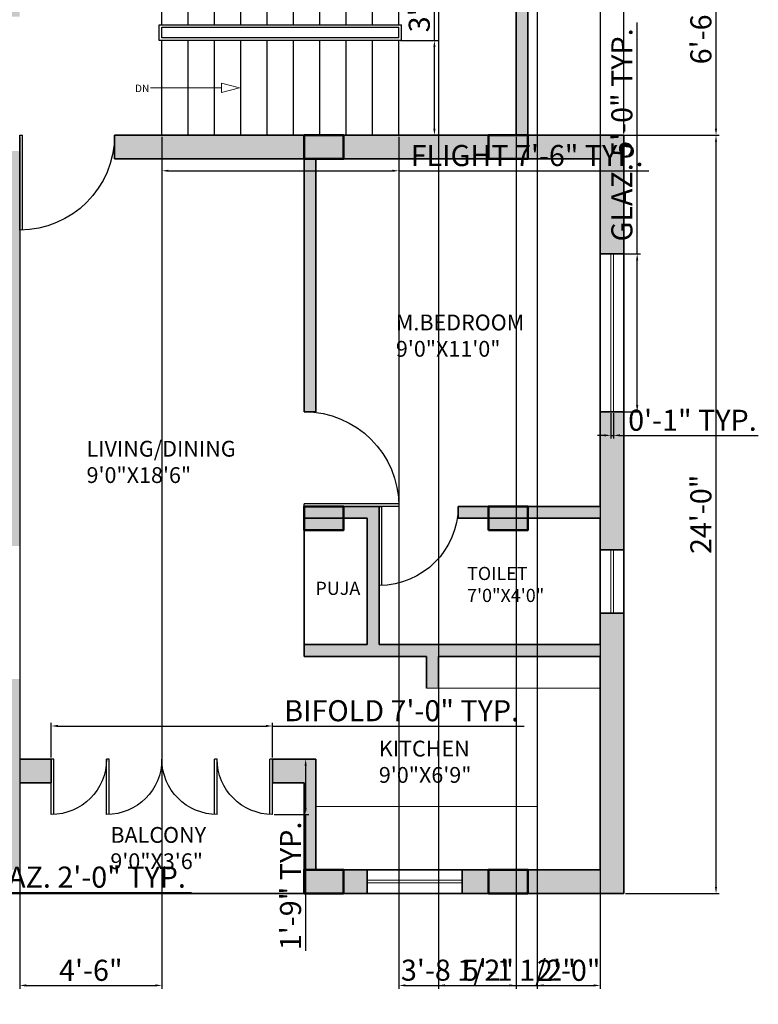
# Model space of a CAD drawing. Units: inches. Extents: x 3010 to 3575, y 2253 to 2995.
# Tile 2 of 4: x 3258 to 3538, y 2253 to 2627. Entities that reach past the tile are written whole.
import ezdxf

# ---------------------------------------------------------------- set-up
doc = ezdxf.new("R2010")
doc.units = ezdxf.units.IN
for name, color, linetype, lineweight in [('A-ANNO-DIMS', 2, 'Continuous', 18), ('A-ANNO-SYMB', 7, 'Continuous', 18), ('A-ANNO-TEXT', 7, 'Continuous', 18), ('A-AREA-IDEN', 7, 'Continuous', 18), ('A-COLS', 7, 'Continuous', 50), ('A-COLS-PATT', 1, 'Continuous', 13), ('A-DOOR', 3, 'Continuous', 25), ('A-FLOR-FIXT', 8, 'Continuous', 18), ('A-FLOR-STRS', 7, 'Continuous', 25), ('A-GLAZ', 4, 'Continuous', 18), ('A-WALL', 7, 'Continuous', 35)]:
    doc.layers.add(name, color=color, linetype=linetype, lineweight=lineweight)
doc.layers.add('A-WALL-PATT', color=9, linetype='Continuous', lineweight=13, true_color=0xc7c8ca)
doc.styles.get("Standard").update_dxf_attribs({"font": 'arial.ttf'})
doc.dimstyles.new('ISO-25', dxfattribs={"dimtxt": 8, "dimasz": 2.5, "dimexe": 1.25, "dimexo": 0.625, "dimtad": 1, "dimdec": 1, "dimlunit": 3, "dimtxsty": 'Standard', "dimcen": 2.5, "dimadec": 0, "dimazin": 0, "dimtfac": 1, "dimtdec": 1, "dimtmove": 0, "dimatfit": 3, "dimfxl": 1, "dimarcsym": 0})

# ---------------------------------------------------------------- blocks, each defined once
blk = doc.blocks.new("D1 3'")
for p, q in [((0, 36), (0, 0)), ((1, 36), (1, 0)), ((0, 0), (1, 0))]:
    blk.add_line(p, q)
blk.add_arc((0, 0), 36, 0, 90)
blk = doc.blocks.new("D2 2'6")
for p, q in [((0, 30), (0, 0)), ((1, 30), (1, 0)), ((0, 0), (1, 0))]:
    blk.add_line(p, q)
blk.add_arc((0, 0), 30, 0, 90)
blk = doc.blocks.new('FLOD D')
for p, q in [((3539.49, 2401.61), (3539.49, 2380.61)), ((3540.49, 2401.61), (3540.49, 2380.61)), ((3560.49, 2401.61), (3560.49, 2380.61)), ((3561.49, 2401.61), (3561.49, 2380.61)), ((3601.49, 2401.61), (3601.49, 2380.61)), ((3602.49, 2401.61), (3602.49, 2380.61)), ((3622.49, 2401.61), (3622.49, 2380.61)), ((3623.49, 2401.61), (3623.49, 2380.61)), ((3540.49, 2380.61), (3539.49, 2380.61)), ((3561.49, 2380.61), (3560.49, 2380.61)), ((3602.49, 2380.61), (3601.49, 2380.61)), ((3623.49, 2380.61), (3622.49, 2380.61))]:
    blk.add_line(p, q)
for centre, start, end in [((3539.49, 2380.61), 0, 90), ((3560.49, 2380.61), 0, 90), ((3602.49, 2380.61), 90, 180), ((3623.49, 2380.61), 90, 180)]:
    blk.add_arc(centre, 21, start, end)
blk = doc.blocks.new('GLAZING-24IN')
for p, q in [((24, 1), (0, 1)), ((24, 0), (0, 0))]:
    blk.add_line(p, q)
blk = doc.blocks.new('GLAZING-36IN')
for p, q in [((36, 1), (0, 1)), ((36, 0), (0, 0))]:
    blk.add_line(p, q)
blk = doc.blocks.new('GLAZING-60IN')
for p, q in [((0, 0), (0, 60)), ((1, 0), (1, 60))]:
    blk.add_line(p, q)
blk = doc.blocks.new('STAIR-FLIGHT-36IN')
for p, q in [((0, 0), (0, 36)), ((10, 0), (10, 36)), ((20, 0), (20, 36)), ((30, 0), (30, 36)), ((40, 0), (40, 36)), ((50, 0), (50, 36)), ((60, 0), (60, 36)), ((70, 0), (70, 36)), ((80, 0), (80, 36)), ((90, 0), (90, 36))]:
    blk.add_line(p, q)
blk = doc.blocks.new('STAIR-DIRECTION-ARROW')
blk.add_line((0, 1.77), (26.94, 1.77))
blk.add_lwpolyline([(33.73, 1.77), (26.94, 3.54), (26.94, 0)], close=True)
blk = doc.blocks.new('KITCHEN-COUNTER-L')
for p, q in [((84, 45), (84, 0)), ((84, 0), (0, 0))]:
    blk.add_line(p, q)
blk = doc.blocks.new('*D17')
at = {"layer": 'A-ANNO-DIMS', "color": 0, "lineweight": -2, "transparency": 16777216}
for p, q in [((3211.45, 2298.76), (3211.45, 2294.53)), ((3235.45, 2298.76), (3235.45, 2294.53)), ((3213.95, 2295.78), (3232.95, 2295.78)), ((3235.45, 2295.78), (3323.23, 2295.78))]:
    blk.add_line(p, q, dxfattribs=at)
at = {"layer": 'A-ANNO-DIMS', "color": 0, "transparency": 16777216}
for points in [[(3213.95, 2296.2), (3213.95, 2295.37), (3211.45, 2295.78)], [(3232.95, 2296.2), (3232.95, 2295.37), (3235.45, 2295.78)]]:
    blk.add_solid(points, dxfattribs=at)
at = {"layer": 'Defpoints', "color": 0, "transparency": 16777216}
for p in [(3211.45, 2299.38), (3235.45, 2299.38), (3235.45, 2295.78)]:
    blk.add_point(p, dxfattribs=at)
at = {"layer": 'A-ANNO-DIMS', "color": 0, "transparency": 16777216, "insert": (3280.59, 2300.54), "char_height": 8, "attachment_point": 5}
blk.add_mtext('GLAZ. 2\'-0" TYP.', dxfattribs=at)
blk = doc.blocks.new('*D21')
at = {"layer": 'A-ANNO-DIMS', "color": 0, "lineweight": -2, "transparency": 16777216}
for p, q in [((3492.45, 2538.38), (3492.45, 2626.17)), ((3484.07, 2538.38), (3493.7, 2538.38)), ((3492.45, 2480.88), (3492.45, 2535.88)), ((3484.07, 2478.38), (3493.7, 2478.38))]:
    blk.add_line(p, q, dxfattribs=at)
at = {"layer": 'A-ANNO-DIMS', "color": 0, "transparency": 16777216}
for points in [[(3492.03, 2535.88), (3492.86, 2535.88), (3492.45, 2538.38)], [(3492.03, 2480.88), (3492.86, 2480.88), (3492.45, 2478.38)]]:
    blk.add_solid(points, dxfattribs=at)
at = {"layer": 'Defpoints', "color": 0, "transparency": 16777216}
for p in [(3483.45, 2538.38), (3492.45, 2538.38), (3483.45, 2478.38)]:
    blk.add_point(p, dxfattribs=at)
at = {"layer": 'A-ANNO-DIMS', "color": 0, "transparency": 16777216, "insert": (3487.68, 2583.52), "char_height": 8, "attachment_point": 5, "rotation": 90}
blk.add_mtext('GLAZ. 5\'-0" TYP.', dxfattribs=at)
blk = doc.blocks.new('*D22')
at = {"layer": 'A-ANNO-DIMS', "color": 0, "lineweight": -2, "transparency": 16777216}
for p, q in [((3482.45, 2477.76), (3482.45, 2468.13)), ((3483.45, 2477.76), (3483.45, 2468.13)), ((3479.95, 2469.38), (3477.45, 2469.38)), ((3482.45, 2469.38), (3483.45, 2469.38)), ((3485.95, 2469.38), (3538.46, 2469.38))]:
    blk.add_line(p, q, dxfattribs=at)
at = {"layer": 'A-ANNO-DIMS', "color": 0, "transparency": 16777216}
for points in [[(3479.95, 2469.8), (3479.95, 2468.97), (3482.45, 2469.38)], [(3485.95, 2469.8), (3485.95, 2468.97), (3483.45, 2469.38)]]:
    blk.add_solid(points, dxfattribs=at)
at = {"layer": 'Defpoints', "color": 0, "transparency": 16777216}
for p in [(3482.45, 2478.38), (3483.45, 2478.38), (3483.45, 2469.38)]:
    blk.add_point(p, dxfattribs=at)
at = {"layer": 'A-ANNO-DIMS', "color": 0, "transparency": 16777216, "insert": (3513.45, 2474.09), "char_height": 8, "attachment_point": 5}
blk.add_mtext('0\'-1" TYP.', dxfattribs=at)
blk = doc.blocks.new('*D29')
at = {"layer": 'A-ANNO-DIMS', "color": 0, "lineweight": -2, "transparency": 16777216}
for p, q in [((3269.95, 2347.01), (3269.95, 2360.23)), ((3353.95, 2347.01), (3353.95, 2360.23)), ((3272.45, 2358.98), (3351.45, 2358.98)), ((3353.95, 2358.98), (3449.58, 2358.98))]:
    blk.add_line(p, q, dxfattribs=at)
at = {"layer": 'A-ANNO-DIMS', "color": 0, "transparency": 16777216}
for points in [[(3272.45, 2359.4), (3272.45, 2358.57), (3269.95, 2358.98)], [(3351.45, 2359.4), (3351.45, 2358.57), (3353.95, 2358.98)]]:
    blk.add_solid(points, dxfattribs=at)
at = {"layer": 'Defpoints', "color": 0, "transparency": 16777216}
for p in [(3353.95, 2358.98), (3269.95, 2346.38), (3353.95, 2346.38)]:
    blk.add_point(p, dxfattribs=at)
at = {"layer": 'A-ANNO-DIMS', "color": 0, "transparency": 16777216, "insert": (3403.01, 2363.75), "char_height": 8, "attachment_point": 5}
blk.add_mtext('BIFOLD 7\'-0" TYP.', dxfattribs=at)
blk = doc.blocks.new('*D30')
at = {"layer": 'A-ANNO-DIMS', "color": 0, "lineweight": -2, "transparency": 16777216}
for p, q in [((3354.57, 2346.38), (3367.8, 2346.38)), ((3366.55, 2343.88), (3366.55, 2327.88)), ((3354.57, 2325.38), (3367.8, 2325.38)), ((3366.55, 2325.38), (3366.55, 2273.62))]:
    blk.add_line(p, q, dxfattribs=at)
at = {"layer": 'A-ANNO-DIMS', "color": 0, "transparency": 16777216}
for points in [[(3366.13, 2343.88), (3366.96, 2343.88), (3366.55, 2346.38)], [(3366.13, 2327.88), (3366.96, 2327.88), (3366.55, 2325.38)]]:
    blk.add_solid(points, dxfattribs=at)
at = {"layer": 'Defpoints', "color": 0, "transparency": 16777216}
for p in [(3353.95, 2346.38), (3353.95, 2325.38), (3366.55, 2325.38)]:
    blk.add_point(p, dxfattribs=at)
at = {"layer": 'A-ANNO-DIMS', "color": 0, "transparency": 16777216, "insert": (3361.84, 2298.25), "char_height": 8, "attachment_point": 5, "rotation": 90}
blk.add_mtext('1\'-9" TYP.', dxfattribs=at)
blk = doc.blocks.new('*D33')
at = {"layer": 'A-ANNO-DIMS', "color": 0, "lineweight": -2, "transparency": 16777216}
for p, q in [((3311.95, 2582.76), (3311.95, 2568.63)), ((3401.95, 2582.76), (3401.95, 2568.63)), ((3314.45, 2569.88), (3399.45, 2569.88)), ((3401.95, 2569.88), (3496.85, 2569.88))]:
    blk.add_line(p, q, dxfattribs=at)
at = {"layer": 'A-ANNO-DIMS', "color": 0, "transparency": 16777216}
for points in [[(3314.45, 2570.3), (3314.45, 2569.47), (3311.95, 2569.88)], [(3399.45, 2570.3), (3399.45, 2569.47), (3401.95, 2569.88)]]:
    blk.add_solid(points, dxfattribs=at)
at = {"layer": 'Defpoints', "color": 0, "transparency": 16777216}
for p in [(3311.95, 2583.38), (3401.95, 2583.38), (3401.95, 2569.88)]:
    blk.add_point(p, dxfattribs=at)
at = {"layer": 'A-ANNO-DIMS', "color": 0, "transparency": 16777216, "insert": (3450.65, 2574.64), "char_height": 8, "attachment_point": 5}
blk.add_mtext('FLIGHT 7\'-6" TYP.', dxfattribs=at)
blk = doc.blocks.new('*D34')
at = {"layer": 'A-ANNO-DIMS', "color": 0, "lineweight": -2, "transparency": 16777216}
for p, q in [((3415.45, 2619.38), (3415.45, 2671.89)), ((3402.57, 2619.38), (3416.7, 2619.38)), ((3415.45, 2585.88), (3415.45, 2616.88)), ((3402.57, 2583.38), (3416.7, 2583.38))]:
    blk.add_line(p, q, dxfattribs=at)
at = {"layer": 'A-ANNO-DIMS', "color": 0, "transparency": 16777216}
for points in [[(3415.03, 2616.88), (3415.86, 2616.88), (3415.45, 2619.38)], [(3415.03, 2585.88), (3415.86, 2585.88), (3415.45, 2583.38)]]:
    blk.add_solid(points, dxfattribs=at)
at = {"layer": 'Defpoints', "color": 0, "transparency": 16777216}
for p in [(3401.95, 2619.38), (3415.45, 2619.38), (3401.95, 2583.38)]:
    blk.add_point(p, dxfattribs=at)
at = {"layer": 'A-ANNO-DIMS', "color": 0, "transparency": 16777216, "insert": (3410.73, 2646.89), "char_height": 8, "attachment_point": 5, "rotation": 90}
blk.add_mtext('3\'-0" TYP.', dxfattribs=at)
blk = doc.blocks.new('*D35')
at = {"layer": 'A-ANNO-DIMS', "color": 0, "lineweight": -2, "transparency": 16777216}
for p, q in [((3257.95, 2582.76), (3257.95, 2259.18)), ((3311.95, 2582.76), (3311.95, 2259.18)), ((3260.45, 2260.43), (3309.45, 2260.43))]:
    blk.add_line(p, q, dxfattribs=at)
at = {"layer": 'A-ANNO-DIMS', "color": 0, "transparency": 16777216}
for points in [[(3260.45, 2260.85), (3260.45, 2260.02), (3257.95, 2260.43)], [(3309.45, 2260.85), (3309.45, 2260.02), (3311.95, 2260.43)]]:
    blk.add_solid(points, dxfattribs=at)
at = {"layer": 'Defpoints', "color": 0, "transparency": 16777216}
for p in [(3257.95, 2583.38), (3311.95, 2583.38), (3311.95, 2260.43)]:
    blk.add_point(p, dxfattribs=at)
at = {"layer": 'A-ANNO-DIMS', "color": 0, "transparency": 16777216, "insert": (3284.95, 2265.14), "char_height": 8, "attachment_point": 5}
blk.add_mtext('4\'-6"', dxfattribs=at)
blk = doc.blocks.new('*D36')
at = {"layer": 'A-ANNO-DIMS', "color": 0, "lineweight": -2, "transparency": 16777216}
for p, q in [((3401.95, 2582.76), (3401.95, 2259.18)), ((3446.45, 2582.76), (3446.45, 2259.18)), ((3404.45, 2260.43), (3443.95, 2260.43))]:
    blk.add_line(p, q, dxfattribs=at)
at = {"layer": 'A-ANNO-DIMS', "color": 0, "transparency": 16777216}
for points in [[(3404.45, 2260.85), (3404.45, 2260.02), (3401.95, 2260.43)], [(3443.95, 2260.85), (3443.95, 2260.02), (3446.45, 2260.43)]]:
    blk.add_solid(points, dxfattribs=at)
at = {"layer": 'Defpoints', "color": 0, "transparency": 16777216}
for p in [(3401.95, 2583.38), (3446.45, 2583.38), (3446.45, 2260.43)]:
    blk.add_point(p, dxfattribs=at)
at = {"layer": 'A-ANNO-DIMS', "color": 0, "transparency": 16777216, "insert": (3424.2, 2265.2), "char_height": 8, "attachment_point": 5}
blk.add_mtext('3\'-8 1/2"', dxfattribs=at)
blk = doc.blocks.new('*D37')
at = {"layer": 'A-ANNO-DIMS', "color": 0, "lineweight": -2, "transparency": 16777216}
for p, q in [((3447.07, 2661.38), (3523.65, 2661.38)), ((3522.4, 2585.88), (3522.4, 2658.88)), ((3447.07, 2583.38), (3523.65, 2583.38))]:
    blk.add_line(p, q, dxfattribs=at)
at = {"layer": 'A-ANNO-DIMS', "color": 0, "transparency": 16777216}
for points in [[(3521.98, 2658.88), (3522.81, 2658.88), (3522.4, 2661.38)], [(3521.98, 2585.88), (3522.81, 2585.88), (3522.4, 2583.38)]]:
    blk.add_solid(points, dxfattribs=at)
at = {"layer": 'Defpoints', "color": 0, "transparency": 16777216}
for p in [(3446.45, 2661.38), (3522.4, 2661.38), (3446.45, 2583.38)]:
    blk.add_point(p, dxfattribs=at)
at = {"layer": 'A-ANNO-DIMS', "color": 0, "transparency": 16777216, "insert": (3517.69, 2622.38), "char_height": 8, "attachment_point": 5, "rotation": 90}
blk.add_mtext('6\'-6"', dxfattribs=at)
blk = doc.blocks.new('*D41')
at = {"layer": 'A-ANNO-DIMS', "color": 0, "lineweight": -2, "transparency": 16777216}
for p, q in [((3454.45, 2693.76), (3454.45, 2259.18)), ((3478.45, 2669.76), (3478.45, 2259.18)), ((3456.95, 2260.43), (3475.95, 2260.43))]:
    blk.add_line(p, q, dxfattribs=at)
at = {"layer": 'A-ANNO-DIMS', "color": 0, "transparency": 16777216}
for points in [[(3456.95, 2260.85), (3456.95, 2260.02), (3454.45, 2260.43)], [(3475.95, 2260.85), (3475.95, 2260.02), (3478.45, 2260.43)]]:
    blk.add_solid(points, dxfattribs=at)
at = {"layer": 'Defpoints', "color": 0, "transparency": 16777216}
for p in [(3454.45, 2694.38), (3478.45, 2670.38), (3478.45, 2260.43)]:
    blk.add_point(p, dxfattribs=at)
at = {"layer": 'A-ANNO-DIMS', "color": 0, "transparency": 16777216, "insert": (3466.45, 2265.14), "char_height": 8, "attachment_point": 5}
blk.add_mtext('2\'-0"', dxfattribs=at)
blk = doc.blocks.new('*D44')
at = {"layer": 'A-ANNO-DIMS', "color": 0, "lineweight": -2, "transparency": 16777216}
for p, q in [((3416.95, 2738.76), (3416.95, 2259.18)), ((3478.45, 2738.76), (3478.45, 2259.18)), ((3419.45, 2260.43), (3475.95, 2260.43))]:
    blk.add_line(p, q, dxfattribs=at)
at = {"layer": 'A-ANNO-DIMS', "color": 0, "transparency": 16777216}
for points in [[(3419.45, 2260.85), (3419.45, 2260.02), (3416.95, 2260.43)], [(3475.95, 2260.85), (3475.95, 2260.02), (3478.45, 2260.43)]]:
    blk.add_solid(points, dxfattribs=at)
at = {"layer": 'Defpoints', "color": 0, "transparency": 16777216}
for p in [(3416.95, 2739.38), (3478.45, 2739.38), (3478.45, 2260.43)]:
    blk.add_point(p, dxfattribs=at)
at = {"layer": 'A-ANNO-DIMS', "color": 0, "transparency": 16777216, "insert": (3447.7, 2265.19), "char_height": 8, "attachment_point": 5}
blk.add_mtext('5\'-1 1/2"', dxfattribs=at)
blk = doc.blocks.new('*D49')
at = {"layer": 'A-ANNO-DIMS', "color": 0, "lineweight": -2, "transparency": 16777216}
for p, q in [((3488.07, 2583.38), (3523.65, 2583.38)), ((3522.4, 2297.88), (3522.4, 2580.88)), ((3488.07, 2295.38), (3523.65, 2295.38))]:
    blk.add_line(p, q, dxfattribs=at)
at = {"layer": 'A-ANNO-DIMS', "color": 0, "transparency": 16777216}
for points in [[(3521.98, 2580.88), (3522.81, 2580.88), (3522.4, 2583.38)], [(3521.98, 2297.88), (3522.81, 2297.88), (3522.4, 2295.38)]]:
    blk.add_solid(points, dxfattribs=at)
at = {"layer": 'Defpoints', "color": 0, "transparency": 16777216}
for p in [(3487.45, 2583.38), (3522.4, 2583.38), (3487.45, 2295.38)]:
    blk.add_point(p, dxfattribs=at)
at = {"layer": 'A-ANNO-DIMS', "color": 0, "transparency": 16777216, "insert": (3517.69, 2439.38), "char_height": 8, "attachment_point": 5, "rotation": 90}
blk.add_mtext('24\'-0"', dxfattribs=at)
blk = doc.blocks.new('*D50')
at = {"layer": 'A-ANNO-DIMS', "color": 0, "lineweight": -2, "transparency": 16777216}
for p, q in [((3450.95, 2584.01), (3450.95, 2979.58)), ((3453.45, 2978.33), (3484.95, 2978.33)), ((3487.45, 2584.01), (3487.45, 2979.58)), ((3487.45, 2978.33), (3531.1, 2978.33))]:
    blk.add_line(p, q, dxfattribs=at)
at = {"layer": 'A-ANNO-DIMS', "color": 0, "transparency": 16777216}
for points in [[(3453.45, 2978.75), (3453.45, 2977.92), (3450.95, 2978.33)], [(3484.95, 2978.75), (3484.95, 2977.92), (3487.45, 2978.33)]]:
    blk.add_solid(points, dxfattribs=at)
at = {"layer": 'Defpoints', "color": 0, "transparency": 16777216}
for p in [(3487.45, 2978.33), (3450.95, 2583.38), (3487.45, 2583.38)]:
    blk.add_point(p, dxfattribs=at)
at = {"layer": 'A-ANNO-DIMS', "color": 0, "transparency": 16777216, "insert": (3510.52, 2983.1), "char_height": 8, "attachment_point": 5}
blk.add_mtext('3\'-0 1/2"', dxfattribs=at)

msp = doc.modelspace()

# ---------------------------------------------------------------- hatches: boundary and pattern name
at = {"layer": 'A-COLS-PATT'}
h = msp.add_hatch(color=256, dxfattribs=at)
h.dxf.hatch_style = 1
h.paths.add_polyline_path([(3380.95, 2574.38), (3380.95, 2583.38), (3365.95, 2583.38), (3365.95, 2574.38)])
h = msp.add_hatch(color=256, dxfattribs=at)
h.dxf.hatch_style = 1
h.paths.add_polyline_path([(3450.95, 2574.38), (3450.95, 2583.38), (3435.95, 2583.38), (3435.95, 2574.38)])
h = msp.add_hatch(color=256, dxfattribs=at)
h.dxf.hatch_style = 1
h.paths.add_polyline_path([(3380.95, 2433.38), (3380.95, 2442.38), (3365.95, 2442.38), (3365.95, 2433.38)])
h = msp.add_hatch(color=256, dxfattribs=at)
h.dxf.hatch_style = 1
h.paths.add_polyline_path([(3450.95, 2433.38), (3450.95, 2442.38), (3435.95, 2442.38), (3435.95, 2433.38)])
h = msp.add_hatch(color=256, dxfattribs=at)
h.dxf.hatch_style = 1
h.paths.add_polyline_path([(3380.95, 2295.38), (3380.95, 2304.38), (3365.95, 2304.38), (3365.95, 2295.38)])
h = msp.add_hatch(color=256, dxfattribs=at)
h.dxf.hatch_style = 1
h.paths.add_polyline_path([(3450.95, 2295.38), (3450.95, 2304.38), (3435.95, 2304.38), (3435.95, 2295.38)])
at = {"layer": 'A-WALL-PATT', "transparency": 33554687}
h = msp.add_hatch(color=256, dxfattribs=at)
h.dxf.hatch_style = 1
h.paths.add_polyline_path([(3064.45, 2499.38), (3055.45, 2499.38), (3055.45, 2457.38), (3064.45, 2457.38)])
h.paths.add_polyline_path([(3091.95, 2421.38), (3055.45, 2421.38), (3055.45, 2382.38), (3064.45, 2382.38), (3064.45, 2412.38), (3091.95, 2412.38)])
h.paths.add_polyline_path([(3248.95, 2421.38), (3176.95, 2421.38), (3176.95, 2464.88), (3194.99, 2464.88), (3194.99, 2473.88), (3176.95, 2473.88), (3176.95, 2551.88), (3172.45, 2551.88), (3172.45, 2515.88), (3172.45, 2421.38), (3106.95, 2421.38), (3106.95, 2412.38), (3248.95, 2412.38)])
h.paths.add_polyline_path([(3064.45, 2346.38), (3055.45, 2346.38), (3055.45, 2295.38), (3091.95, 2295.38), (3091.95, 2304.38), (3064.45, 2304.38)])
h.paths.add_polyline_path([(3129.95, 2304.38), (3106.95, 2304.38), (3106.95, 2295.38), (3129.95, 2295.38)])
h.paths.add_polyline_path([(3211.45, 2304.38), (3193.45, 2304.38), (3193.45, 2376.88), (3188.95, 2376.88), (3188.95, 2304.38), (3165.95, 2304.38), (3165.95, 2295.38), (3211.45, 2295.38)])
h.paths.add_polyline_path([(3269.95, 2346.38), (3257.95, 2346.38), (3257.95, 2376.88), (3223.45, 2376.88), (3223.45, 2371.88), (3253.45, 2371.88), (3253.45, 2304.38), (3257.95, 2304.38), (3257.95, 2337.38), (3269.95, 2337.38)])
h.paths.add_polyline_path([(3242.95, 2304.38), (3235.45, 2304.38), (3235.45, 2295.38), (3242.95, 2295.38)])
h.paths.add_polyline_path([(3370.45, 2346.38), (3353.95, 2346.38), (3353.95, 2337.38), (3365.95, 2337.38), (3365.95, 2304.38), (3370.45, 2304.38)])
h.paths.add_polyline_path([(3389.94, 2304.38), (3380.95, 2304.38), (3380.95, 2295.38), (3389.94, 2295.38)], flags=17)
h.paths.add_polyline_path([(3435.95, 2304.38), (3425.94, 2304.38), (3425.94, 2295.38), (3435.95, 2295.38)], flags=17)
h.paths.add_polyline_path([(3487.45, 2401.88), (3478.45, 2401.88), (3478.45, 2389.88), (3394.45, 2389.88), (3394.45, 2442.38), (3380.95, 2442.38), (3380.95, 2437.88), (3389.95, 2437.88), (3389.95, 2389.88), (3365.95, 2389.88), (3365.95, 2385.38), (3412.45, 2385.38), (3412.45, 2373.38), (3416.95, 2373.38), (3416.95, 2385.38), (3478.45, 2385.38), (3478.45, 2304.38), (3450.95, 2304.38), (3450.95, 2295.38), (3487.45, 2295.38)])
h.paths.add_polyline_path([(3487.45, 2478.38), (3478.45, 2478.38), (3478.45, 2442.38), (3450.95, 2442.38), (3450.95, 2437.88), (3478.45, 2437.88), (3478.45, 2425.88), (3487.45, 2425.88)])
h.paths.add_polyline_path([(3435.95, 2442.38), (3424.45, 2442.38), (3424.45, 2437.88), (3435.95, 2437.88)], flags=17)
h.paths.add_polyline_path([(3248.95, 2592.38), (3221.95, 2592.38), (3172.45, 2592.38), (3172.45, 2587.88), (3248.95, 2587.88)])
h.paths.add_polyline_path([(3257.95, 2577.38), (3248.95, 2577.38), (3248.95, 2473.88), (3230.99, 2473.88), (3230.99, 2464.88), (3248.95, 2464.88), (3248.95, 2427.38), (3257.95, 2427.38)])
h.paths.add_polyline_path([(3365.95, 2583.38), (3293.95, 2583.38), (3293.95, 2574.38), (3365.95, 2574.38)])
h.paths.add_polyline_path([(3370.45, 2574.38), (3365.95, 2574.38), (3365.95, 2478.38), (3370.45, 2478.38)])
h.paths.add_polyline_path([(3435.95, 2583.38), (3380.95, 2583.38), (3380.95, 2574.38), (3435.95, 2574.38)])
h.paths.add_polyline_path([(3487.45, 2583.38), (3450.95, 2583.38), (3450.95, 2574.38), (3478.45, 2574.38), (3478.45, 2538.38), (3487.45, 2538.38)])
h.paths.add_polyline_path([(3064.45, 2551.88), (3055.45, 2551.88), (3055.45, 2535.38), (3136.45, 2535.38), (3136.45, 2557.88), (3131.95, 2557.88), (3131.95, 2539.88), (3064.45, 2539.88)])
h.paths.add_polyline_path([(3091.95, 2704.88), (3064.45, 2704.88), (3064.45, 2726.63), (3055.45, 2726.63), (3055.45, 2676.38), (3064.45, 2676.38), (3064.45, 2700.38), (3091.95, 2700.38)])
h.paths.add_polyline_path([(3064.45, 2616.38), (3055.45, 2616.38), (3055.45, 2575.88), (3064.45, 2575.88), (3064.45, 2587.88), (3091.95, 2587.88), (3091.95, 2592.38), (3064.45, 2592.38)])
h.paths.add_polyline_path([(3487.45, 2688.38), (3478.45, 2688.38), (3478.45, 2670.38), (3450.95, 2670.38), (3450.95, 2661.38), (3487.45, 2661.38)])
h.paths.add_polyline_path([(3450.95, 2661.38), (3446.45, 2661.38), (3446.45, 2583.38), (3450.95, 2583.38)])
h.paths.add_polyline_path([(3435.95, 2670.38), (3380.95, 2670.38), (3380.95, 2661.38), (3435.95, 2661.38)])
h.paths.add_polyline_path([(3365.95, 2670.38), (3293.95, 2670.38), (3293.95, 2661.38), (3365.95, 2661.38)])
h.paths.add_polyline_path([(3370.45, 2715.38), (3365.95, 2715.38), (3365.95, 2670.38), (3370.45, 2670.38)])
h.paths.add_polyline_path([(3257.95, 2700.38), (3248.95, 2700.38), (3248.95, 2628.38), (3257.95, 2628.38)])
h.paths.add_polyline_path([(3128.95, 2742.38), (3124.45, 2742.38), (3124.45, 2704.88), (3106.95, 2704.88), (3106.95, 2700.38), (3128.95, 2700.38)])
h.paths.add_polyline_path([(3248.95, 2704.88), (3164.95, 2704.88), (3164.95, 2700.38), (3248.95, 2700.38)])
h.paths.add_polyline_path([(3257.95, 2817.38), (3248.95, 2817.38), (3248.95, 2715.38), (3257.95, 2715.38)])
h.paths.add_polyline_path([(3128.95, 2781.38), (3055.45, 2781.38), (3055.45, 2750.63), (3064.45, 2750.63), (3064.45, 2772.38), (3128.95, 2772.38)])
h.paths.add_polyline_path([(3242.95, 2826.38), (3106.95, 2826.38), (3106.95, 2817.38), (3242.95, 2817.38)])
h.paths.add_polyline_path([(3091.95, 2826.38), (3064.45, 2826.38), (3064.45, 2856.38), (3055.45, 2856.38), (3055.45, 2817.38), (3091.95, 2817.38)])
h.paths.add_polyline_path([(3064.45, 2934.38), (3091.95, 2934.38), (3091.95, 2943.38), (3055.45, 2943.38), (3055.45, 2904.38), (3064.45, 2904.38)])
h.paths.add_polyline_path([(3140.95, 2943.38), (3106.95, 2943.38), (3106.95, 2934.38), (3140.95, 2934.38)])
h.paths.add_polyline_path([(3211.45, 2943.38), (3188.95, 2943.38), (3188.95, 2862.38), (3223.45, 2862.38), (3223.45, 2866.88), (3193.45, 2866.88), (3193.45, 2934.38), (3211.45, 2934.38)])
h.paths.add_polyline_path([(3257.95, 2934.38), (3253.45, 2934.38), (3253.45, 2862.38), (3257.95, 2862.38), (3257.95, 2892.38), (3269.95, 2892.38), (3269.95, 2901.38), (3257.95, 2901.38)])
h.paths.add_polyline_path([(3242.95, 2943.38), (3235.45, 2943.38), (3235.45, 2934.38), (3242.95, 2934.38)])
h.paths.add_polyline_path([(3370.45, 2934.38), (3365.95, 2934.38), (3365.95, 2901.38), (3353.95, 2901.38), (3353.95, 2892.38), (3365.95, 2892.38), (3365.95, 2844.38), (3370.45, 2844.38)])
h.paths.add_polyline_path([(3389.94, 2943.38), (3380.95, 2943.38), (3380.95, 2934.38), (3389.94, 2934.38)])
h.paths.add_polyline_path([(3435.95, 2943.38), (3425.94, 2943.38), (3425.94, 2934.38), (3435.95, 2934.38)])
h.paths.add_polyline_path([(3487.45, 2943.38), (3450.95, 2943.38), (3450.95, 2934.38), (3478.45, 2934.38), (3478.45, 2895.38), (3487.45, 2895.38)])
h.paths.add_polyline_path([(3487.45, 2847.38), (3478.45, 2847.38), (3478.45, 2808.38), (3450.95, 2808.38), (3450.95, 2803.88), (3478.45, 2803.88), (3478.45, 2791.88), (3487.45, 2791.88)])
h.paths.add_polyline_path([(3435.95, 2808.38), (3424.45, 2808.38), (3424.45, 2803.88), (3435.95, 2803.88)])
h.paths.add_polyline_path([(3487.45, 2767.88), (3478.45, 2767.88), (3478.45, 2755.88), (3394.45, 2755.88), (3394.45, 2808.38), (3380.95, 2808.38), (3380.95, 2803.88), (3389.95, 2803.88), (3389.95, 2755.88), (3365.95, 2755.88), (3365.95, 2751.38), (3412.45, 2751.38), (3412.45, 2739.38), (3416.95, 2739.38), (3416.95, 2751.38), (3478.45, 2751.38), (3478.45, 2724.38), (3487.45, 2724.38)])
h.paths.add_polyline_path([(3398.97, 2495.84), (3456.57, 2495.84), (3456.57, 2518.66), (3398.97, 2518.66)], flags=9)

# ---------------------------------------------------------------- linework, layer by layer
at = {"layer": 'A-COLS'}
for points in [[(3365.95, 2574.38), (3365.95, 2583.38), (3380.95, 2583.38), (3380.95, 2574.38)], [(3435.95, 2574.38), (3435.95, 2583.38), (3450.95, 2583.38), (3450.95, 2574.38)], [(3365.95, 2433.38), (3365.95, 2442.38), (3380.95, 2442.38), (3380.95, 2433.38)], [(3435.95, 2433.38), (3435.95, 2442.38), (3450.95, 2442.38), (3450.95, 2433.38)], [(3365.95, 2295.38), (3365.95, 2304.38), (3380.95, 2304.38), (3380.95, 2295.38)], [(3435.95, 2295.38), (3435.95, 2304.38), (3450.95, 2304.38), (3450.95, 2295.38)]]:
    msp.add_lwpolyline(points, close=True, dxfattribs=at)
at = {"layer": 'A-FLOR-FIXT'}
msp.add_line((3478.45, 2373.38), (3412.45, 2373.38), dxfattribs=at)
at = {"layer": 'A-FLOR-STRS'}
for p, q in [((3310.95, 2625.38), (3402.95, 2625.38)), ((3310.95, 2619.38), (3310.95, 2625.38)), ((3311.95, 2624.38), (3401.95, 2624.38)), ((3311.95, 2620.38), (3311.95, 2624.38)), ((3401.95, 2620.38), (3401.95, 2624.38)), ((3402.95, 2619.38), (3402.95, 2625.38)), ((3402.95, 2619.38), (3310.95, 2619.38)), ((3401.95, 2620.38), (3311.95, 2620.38))]:
    msp.add_line(p, q, dxfattribs=at)
at = {"layer": 'A-WALL'}
for p, q in [((3446.45, 2583.38), (3446.45, 2661.38)), ((3450.95, 2583.38), (3450.95, 2661.38)), ((3293.95, 2574.38), (3293.95, 2583.38)), ((3487.45, 2583.38), (3293.95, 2583.38)), ((3487.45, 2583.38), (3487.45, 2295.38)), ((3365.95, 2574.38), (3293.95, 2574.38)), ((3365.95, 2574.38), (3365.95, 2478.38)), ((3478.45, 2574.38), (3370.45, 2574.38)), ((3370.45, 2574.38), (3370.45, 2478.38)), ((3478.45, 2574.38), (3478.45, 2442.38)), ((3487.45, 2538.38), (3478.45, 2538.38)), ((3370.45, 2478.38), (3365.95, 2478.38)), ((3487.45, 2478.38), (3478.45, 2478.38)), ((3365.95, 2442.38), (3365.95, 2385.38)), ((3394.45, 2442.38), (3365.95, 2442.38)), ((3394.45, 2442.38), (3394.45, 2389.88)), ((3478.45, 2442.38), (3424.45, 2442.38)), ((3424.45, 2442.38), (3424.45, 2437.88)), ((3389.95, 2437.88), (3365.95, 2437.88)), ((3389.95, 2437.88), (3389.95, 2389.88)), ((3478.45, 2437.88), (3424.45, 2437.88)), ((3478.45, 2437.88), (3478.45, 2389.88)), ((3487.45, 2425.88), (3478.45, 2425.88)), ((3487.45, 2401.88), (3478.45, 2401.88)), ((3389.95, 2389.88), (3365.95, 2389.88)), ((3478.45, 2389.88), (3394.45, 2389.88)), ((3412.45, 2385.38), (3365.95, 2385.38)), ((3412.45, 2385.38), (3412.45, 2373.38)), ((3478.45, 2385.38), (3416.95, 2385.38)), ((3416.95, 2385.38), (3416.95, 2373.38)), ((3478.45, 2385.38), (3478.45, 2304.38)), ((3269.95, 2346.38), (3257.95, 2346.38)), ((3269.95, 2337.38), (3269.95, 2346.38)), ((3370.45, 2346.38), (3353.95, 2346.38)), ((3353.95, 2346.38), (3353.95, 2337.38)), ((3370.45, 2346.38), (3370.45, 2304.38)), ((3269.95, 2337.38), (3257.95, 2337.38)), ((3365.95, 2337.38), (3353.95, 2337.38)), ((3365.95, 2337.38), (3365.95, 2295.38)), ((3478.45, 2304.38), (3370.45, 2304.38)), ((3389.94, 2304.38), (3389.94, 2295.38)), ((3425.94, 2304.38), (3425.94, 2295.38)), ((3487.45, 2295.38), (3055.45, 2295.38))]:
    msp.add_line(p, q, dxfattribs=at)

# ---------------------------------------------------------------- block references
at = {"layer": 'A-ANNO-SYMB'}
msp.add_blockref('STAIR-DIRECTION-ARROW', (3307.68, 2599.61), dxfattribs=at)
at = {"layer": 'A-DOOR', "xscale": -1}
for name, p, rotation in [("D1 3'", (3257.95, 2583.38), 180), ("D1 3'", (3365.95, 2442.38), 270), ("D2 2'6", (3394.45, 2442.38), 180), ('FLOD D', (-269.55, 4726.99), 180)]:
    msp.add_blockref(name, p, dxfattribs=dict(at, rotation=rotation))
at = {"layer": 'A-FLOR-FIXT'}
msp.add_blockref('KITCHEN-COUNTER-L', (3370.45, 2328.38), dxfattribs=at)
at = {"layer": 'A-FLOR-STRS'}
for p in [(3311.95, 2625.38), (3311.95, 2583.38)]:
    msp.add_blockref('STAIR-FLIGHT-36IN', p, dxfattribs=at)
at = {"layer": 'A-GLAZ'}
for name, p in [('GLAZING-60IN', (3482.45, 2478.38)), ('GLAZING-36IN', (3389.94, 2299.38))]:
    msp.add_blockref(name, p, dxfattribs=at)
at = {"layer": 'A-GLAZ', "rotation": 270.0000000000001}
msp.add_blockref('GLAZING-24IN', (3482.45, 2425.88), dxfattribs=at)

# ---------------------------------------------------------------- texts
at = {"layer": 'A-ANNO-TEXT'}
msp.add_text('DN', height=2.842, dxfattribs=at).set_placement((3301.71, 2599.77))
at = {"layer": 'A-AREA-IDEN', "attachment_point": 1}
for s, insert, char_height in [('{\\fTimes New Roman|b0|i0|c0|p18;\\PM.BEDROOM \\P9\'0"X11\'0"}', (3400.82, 2525.26), 6), ('{\\fTimes New Roman|b0|i0|c0|p18;\\PLIVING/DINING\\P9\'0"X18\'6"}', (3283.34, 2477.3), 6), ('{\\fTimes New Roman|b0|i0|c0|p18;\\P  TOILET\\P  7\'0"X4\'0"}', (3424.8, 2427.75), 5), ('{\\fTimes New Roman|b0|i0|c0|p18;\\PPUJA}', (3370.26, 2422.12), 5), ('{\\fTimes New Roman|b0|i0|c0|p18;\\PKITCHEN\\P9\'0"X6\'9"}', (3394.35, 2363.4), 6), ('{\\fTimes New Roman|b0|i0|c0|p18;\\PBALCONY \\P9\'0"X3\'6"}', (3292.38, 2330.61), 6)]:
    msp.add_mtext_dynamic_manual_height_columns(s, width=72.5587, gutter_width=12.5, heights=[0], dxfattribs=dict(at, insert=insert, char_height=char_height))

# ---------------------------------------------------------------- dimensions: what is measured, and where the dimension line sits
at = {"layer": 'A-ANNO-DIMS'}
for base, p1, p2, picture, middle in [((3487.45, 2978.33), (3450.95, 2583.38), (3487.45, 2583.38), '*D50', (3510.52, 2983.1)), ((3478.45, 2260.43), (3416.95, 2739.38), (3478.45, 2739.38), '*D44', (3447.7, 2265.19)), ((3478.45, 2260.43), (3454.45, 2694.38), (3478.45, 2670.38), '*D41', (3466.45, 2265.14)), ((3311.95, 2260.43), (3257.95, 2583.38), (3311.95, 2583.38), '*D35', (3284.95, 2265.14)), ((3446.45, 2260.43), (3401.95, 2583.38), (3446.45, 2583.38), '*D36', (3424.2, 2265.2))]:
    dim = msp.add_linear_dim(base=base, p1=p1, p2=p2, dimstyle='ISO-25', override={"dimdec": 1, "dimlfac": 1, "dimrnd": 0, "dimzin": 1, "dimdsep": 46, "dimlunit": 4, "dimfrac": 2}, dxfattribs=at)
    dim.commit()
    dim.dimension.update_dxf_attribs({"geometry": picture, "text_midpoint": middle})
for base, p1, p2, angle, text, picture, middle in [((3415.45, 2619.38), (3401.95, 2583.38), (3401.95, 2619.38), 90, '<> TYP.', '*D34', (3410.73, 2646.89)), ((3492.45, 2538.38), (3483.45, 2478.38), (3483.45, 2538.38), 90, 'GLAZ. <> TYP.', '*D21', (3487.68, 2583.52)), ((3366.55, 2325.38), (3353.95, 2346.38), (3353.95, 2325.38), 270, '<> TYP.', '*D30', (3361.84, 2298.25))]:
    dim = msp.add_linear_dim(base=base, p1=p1, p2=p2, angle=angle, text=text, dimstyle='ISO-25', override={"dimdec": 1, "dimlfac": 1, "dimrnd": 0, "dimzin": 1, "dimdsep": 46, "dimlunit": 4, "dimfrac": 2}, dxfattribs=at)
    dim.commit()
    dim.dimension.update_dxf_attribs({"geometry": picture, "text_midpoint": middle})
for base, p1, p2, picture, middle in [((3522.4, 2661.38), (3446.45, 2583.38), (3446.45, 2661.38), '*D37', (3517.69, 2622.38)), ((3522.4, 2583.38), (3487.45, 2295.38), (3487.45, 2583.38), '*D49', (3517.69, 2439.38))]:
    dim = msp.add_linear_dim(base=base, p1=p1, p2=p2, angle=90, dimstyle='ISO-25', override={"dimdec": 1, "dimlfac": 1, "dimrnd": 0, "dimzin": 1, "dimdsep": 46, "dimlunit": 4, "dimfrac": 2}, dxfattribs=at)
    dim.commit()
    dim.dimension.update_dxf_attribs({"geometry": picture, "text_midpoint": middle})
for base, p1, p2, text, picture, middle in [((3401.95, 2569.88), (3311.95, 2583.38), (3401.95, 2583.38), 'FLIGHT <> TYP.', '*D33', (3450.65, 2574.64)), ((3483.45, 2469.38), (3482.45, 2478.38), (3483.45, 2478.38), '<> TYP.', '*D22', (3513.45, 2474.09)), ((3353.95, 2358.98), (3269.95, 2346.38), (3353.95, 2346.38), 'BIFOLD <> TYP.', '*D29', (3403.01, 2363.75)), ((3235.45, 2295.78), (3211.45, 2299.38), (3235.45, 2299.38), 'GLAZ. <> TYP.', '*D17', (3280.59, 2300.54))]:
    dim = msp.add_linear_dim(base=base, p1=p1, p2=p2, text=text, dimstyle='ISO-25', override={"dimdec": 1, "dimlfac": 1, "dimrnd": 0, "dimzin": 1, "dimdsep": 46, "dimlunit": 4, "dimfrac": 2}, dxfattribs=at)
    dim.commit()
    dim.dimension.update_dxf_attribs({"geometry": picture, "text_midpoint": middle})

doc.saveas('drawing.dxf')
